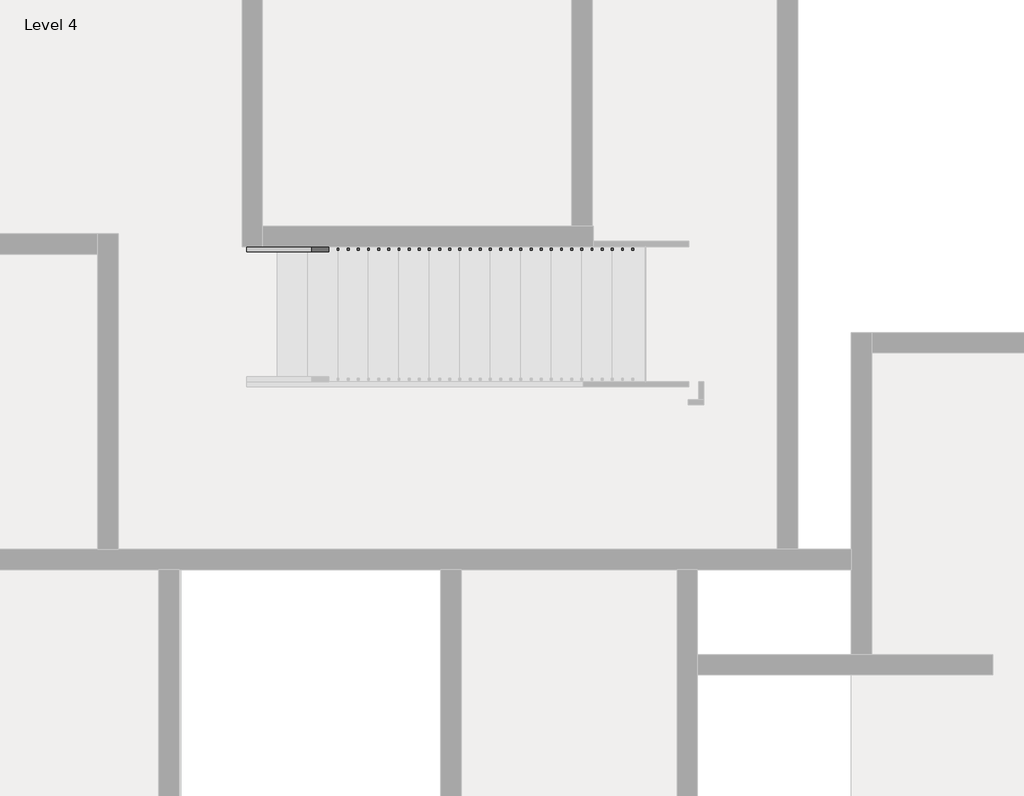
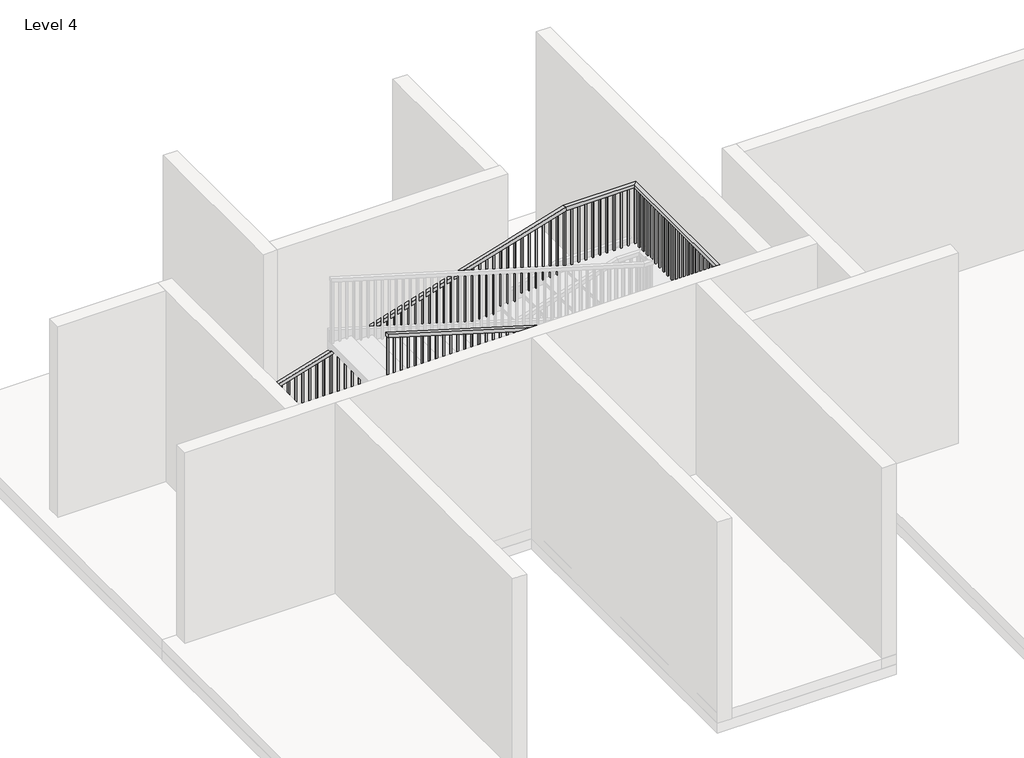
# One storey, part 10 of 14: 1 railing.
"""IFC4 building model written with IfcOpenShell, lengths in millimetres."""

from ifc_helpers import new_model, si_unit, frame, origin, place, context, project, spatial, polyline, outline, extrude, faceted_brep, element, save

model = new_model("IFC4")

# Units and contexts
model_context = context("Model", 3, world=origin())
ifc_project = project(units=[si_unit("LENGTHUNIT", "METRE", prefix="MILLI")], contexts=[model_context])

# Site, building, storey
site = spatial("IfcSite", under=ifc_project)
building = spatial("IfcBuilding", under=site)
storey = spatial("IfcBuildingStorey", under=building, Name="Level 4", Elevation=9144.0)

# Railing
placement = place(None, origin())
element("IfcRailing", 1, ObjectType="Handrail - Rectangular", at=placement, inside=storey, context=model_context, shape_type="SolidModel", body=[
    faceted_brep([(-5254.0891351, 12506.0715905, 10149.84), (-5254.0891351, 12506.0715905, 10096.8032429), (-5254.0891351, 12455.2715905, 10096.8032429), (-5254.0891351, 12455.2715905, 10149.84), (-986.8891351, 12506.0715905, 11430.0), (-979.4332782, 12506.0715905, 11379.2), (-979.4332782, 12455.2715905, 11379.2), (-986.8891351, 12455.2715905, 11430.0), (54.5108649, 12506.0715905, 11430.0), (54.5108649, 12506.0715905, 11379.2), (3.7108649, 12455.2715905, 11379.2), (3.7108649, 12455.2715905, 11430.0), (54.5108649, 9478.4949943, 11430.0), (54.5108649, 9478.4949943, 11379.2), (3.7108649, 9529.2949943, 11379.2), (3.7108649, 9529.2949943, 11430.0), (-682.0891351, 9478.4949943, 11430.0), (-689.544992, 9478.4949943, 11379.2), (-689.544992, 9529.2949943, 11379.2), (-682.0891351, 9529.2949943, 11430.0), (-5254.0891351, 9478.4949943, 12801.6), (-5254.0891351, 9529.2949943, 12801.6), (-5254.0891351, 9529.2949943, 12748.5632429), (-5254.0891351, 9478.4949943, 12748.5632429)], [[[0, 1, 2, 3]], [[1, 0, 4, 5]], [[2, 1, 5, 6]], [[3, 2, 6, 7]], [[0, 3, 7, 4]], [[5, 4, 8, 9]], [[6, 5, 9, 10]], [[7, 6, 10, 11]], [[4, 7, 11, 8]], [[9, 8, 12, 13]], [[10, 9, 13, 14]], [[11, 10, 14, 15]], [[8, 11, 15, 12]], [[13, 12, 16, 17]], [[14, 13, 17, 18]], [[15, 14, 18, 19]], [[12, 15, 19, 16]], [[20, 21, 22, 23]], [[17, 16, 20, 23]], [[18, 17, 23, 22]], [[19, 18, 22, 21]], [[16, 19, 21, 20]]]),
    extrude(outline(polyline([(12720.9407429, -5162.0141351), (11795.76, -5162.0141351), (11795.76, -5142.9641351), (12715.2257429, -5142.9641351), (12720.9407429, -5162.0141351)])), frame((0.0, 9494.3699943, 0.0), z_axis=(0.0, 1.0, 0.0), x_axis=(0.0, 0.0, 1.0)), (0.0, 0.0, 1.0), 19.05),
    extrude(outline(polyline([(12690.4607429, -5060.4141351), (11795.76, -5060.4141351), (11795.76, -5041.3641351), (12684.7457429, -5041.3641351), (12690.4607429, -5060.4141351)])), frame((0.0, 9494.3699943, 0.0), z_axis=(0.0, 1.0, 0.0), x_axis=(0.0, 0.0, 1.0)), (0.0, 0.0, 1.0), 19.05),
    extrude(outline(polyline([(12659.9807429, -4958.8141351), (11795.76, -4958.8141351), (11795.76, -4939.7641351), (12654.2657429, -4939.7641351), (12659.9807429, -4958.8141351)])), frame((0.0, 9494.3699943, 0.0), z_axis=(0.0, 1.0, 0.0), x_axis=(0.0, 0.0, 1.0)), (0.0, 0.0, 1.0), 19.05),
    extrude(outline(polyline([(12629.5007429, -4857.2141351), (11704.32, -4857.2141351), (11704.32, -4838.1641351), (12623.7857429, -4838.1641351), (12629.5007429, -4857.2141351)])), frame((0.0, 9494.3699943, 0.0), z_axis=(0.0, 1.0, 0.0), x_axis=(0.0, 0.0, 1.0)), (0.0, 0.0, 1.0), 19.05),
    extrude(outline(polyline([(12599.0207429, -4755.6141351), (11704.32, -4755.6141351), (11704.32, -4736.5641351), (12593.3057429, -4736.5641351), (12599.0207429, -4755.6141351)])), frame((0.0, 9494.3699943, 0.0), z_axis=(0.0, 1.0, 0.0), x_axis=(0.0, 0.0, 1.0)), (0.0, 0.0, 1.0), 19.05),
    extrude(outline(polyline([(12568.5407429, -4654.0141351), (11704.32, -4654.0141351), (11704.32, -4634.9641351), (12562.8257429, -4634.9641351), (12568.5407429, -4654.0141351)])), frame((0.0, 9494.3699943, 0.0), z_axis=(0.0, 1.0, 0.0), x_axis=(0.0, 0.0, 1.0)), (0.0, 0.0, 1.0), 19.05),
    extrude(outline(polyline([(12538.0607429, -4552.4141351), (11612.88, -4552.4141351), (11612.88, -4533.3641351), (12532.3457429, -4533.3641351), (12538.0607429, -4552.4141351)])), frame((0.0, 9494.3699943, 0.0), z_axis=(0.0, 1.0, 0.0), x_axis=(0.0, 0.0, 1.0)), (0.0, 0.0, 1.0), 19.05),
    extrude(outline(polyline([(12507.5807429, -4450.8141351), (11612.88, -4450.8141351), (11612.88, -4431.7641351), (12501.8657429, -4431.7641351), (12507.5807429, -4450.8141351)])), frame((0.0, 9494.3699943, 0.0), z_axis=(0.0, 1.0, 0.0), x_axis=(0.0, 0.0, 1.0)), (0.0, 0.0, 1.0), 19.05),
    extrude(outline(polyline([(12477.1007429, -4349.2141351), (11612.88, -4349.2141351), (11612.88, -4330.1641351), (12471.3857429, -4330.1641351), (12477.1007429, -4349.2141351)])), frame((0.0, 9494.3699943, 0.0), z_axis=(0.0, 1.0, 0.0), x_axis=(0.0, 0.0, 1.0)), (0.0, 0.0, 1.0), 19.05),
    extrude(outline(polyline([(12446.6207429, -4247.6141351), (11521.44, -4247.6141351), (11521.44, -4228.5641351), (12440.9057429, -4228.5641351), (12446.6207429, -4247.6141351)])), frame((0.0, 9494.3699943, 0.0), z_axis=(0.0, 1.0, 0.0), x_axis=(0.0, 0.0, 1.0)), (0.0, 0.0, 1.0), 19.05),
    extrude(outline(polyline([(12416.1407429, -4146.0141351), (11521.44, -4146.0141351), (11521.44, -4126.9641351), (12410.4257429, -4126.9641351), (12416.1407429, -4146.0141351)])), frame((0.0, 9494.3699943, 0.0), z_axis=(0.0, 1.0, 0.0), x_axis=(0.0, 0.0, 1.0)), (0.0, 0.0, 1.0), 19.05),
    extrude(outline(polyline([(12385.6607429, -4044.4141351), (11521.44, -4044.4141351), (11521.44, -4025.3641351), (12379.9457429, -4025.3641351), (12385.6607429, -4044.4141351)])), frame((0.0, 9494.3699943, 0.0), z_axis=(0.0, 1.0, 0.0), x_axis=(0.0, 0.0, 1.0)), (0.0, 0.0, 1.0), 19.05),
    extrude(outline(polyline([(12355.1807429, -3942.8141351), (11430.0, -3942.8141351), (11430.0, -3923.7641351), (12349.4657429, -3923.7641351), (12355.1807429, -3942.8141351)])), frame((0.0, 9494.3699943, 0.0), z_axis=(0.0, 1.0, 0.0), x_axis=(0.0, 0.0, 1.0)), (0.0, 0.0, 1.0), 19.05),
    extrude(outline(polyline([(12324.7007429, -3841.2141351), (11430.0, -3841.2141351), (11430.0, -3822.1641351), (12318.9857429, -3822.1641351), (12324.7007429, -3841.2141351)])), frame((0.0, 9494.3699943, 0.0), z_axis=(0.0, 1.0, 0.0), x_axis=(0.0, 0.0, 1.0)), (0.0, 0.0, 1.0), 19.05),
    extrude(outline(polyline([(12294.2207429, -3739.6141351), (11430.0, -3739.6141351), (11430.0, -3720.5641351), (12288.5057429, -3720.5641351), (12294.2207429, -3739.6141351)])), frame((0.0, 9494.3699943, 0.0), z_axis=(0.0, 1.0, 0.0), x_axis=(0.0, 0.0, 1.0)), (0.0, 0.0, 1.0), 19.05),
    extrude(outline(polyline([(12263.7407429, -3638.0141351), (11338.56, -3638.0141351), (11338.56, -3618.9641351), (12258.0257429, -3618.9641351), (12263.7407429, -3638.0141351)])), frame((0.0, 9494.3699943, 0.0), z_axis=(0.0, 1.0, 0.0), x_axis=(0.0, 0.0, 1.0)), (0.0, 0.0, 1.0), 19.05),
    extrude(outline(polyline([(12233.2607429, -3536.4141351), (11338.56, -3536.4141351), (11338.56, -3517.3641351), (12227.5457429, -3517.3641351), (12233.2607429, -3536.4141351)])), frame((0.0, 9494.3699943, 0.0), z_axis=(0.0, 1.0, 0.0), x_axis=(0.0, 0.0, 1.0)), (0.0, 0.0, 1.0), 19.05),
    extrude(outline(polyline([(12202.7807429, -3434.8141351), (11338.56, -3434.8141351), (11338.56, -3415.7641351), (12197.0657429, -3415.7641351), (12202.7807429, -3434.8141351)])), frame((0.0, 9494.3699943, 0.0), z_axis=(0.0, 1.0, 0.0), x_axis=(0.0, 0.0, 1.0)), (0.0, 0.0, 1.0), 19.05),
    extrude(outline(polyline([(12172.3007429, -3333.2141351), (11247.12, -3333.2141351), (11247.12, -3314.1641351), (12166.5857429, -3314.1641351), (12172.3007429, -3333.2141351)])), frame((0.0, 9494.3699943, 0.0), z_axis=(0.0, 1.0, 0.0), x_axis=(0.0, 0.0, 1.0)), (0.0, 0.0, 1.0), 19.05),
    extrude(outline(polyline([(12141.8207429, -3231.6141351), (11247.12, -3231.6141351), (11247.12, -3212.5641351), (12136.1057429, -3212.5641351), (12141.8207429, -3231.6141351)])), frame((0.0, 9494.3699943, 0.0), z_axis=(0.0, 1.0, 0.0), x_axis=(0.0, 0.0, 1.0)), (0.0, 0.0, 1.0), 19.05),
    extrude(outline(polyline([(12111.3407429, -3130.0141351), (11247.12, -3130.0141351), (11247.12, -3110.9641351), (12105.6257429, -3110.9641351), (12111.3407429, -3130.0141351)])), frame((0.0, 9494.3699943, 0.0), z_axis=(0.0, 1.0, 0.0), x_axis=(0.0, 0.0, 1.0)), (0.0, 0.0, 1.0), 19.05),
    extrude(outline(polyline([(12080.8607429, -3028.4141351), (11155.68, -3028.4141351), (11155.68, -3009.3641351), (12075.1457429, -3009.3641351), (12080.8607429, -3028.4141351)])), frame((0.0, 9494.3699943, 0.0), z_axis=(0.0, 1.0, 0.0), x_axis=(0.0, 0.0, 1.0)), (0.0, 0.0, 1.0), 19.05),
    extrude(outline(polyline([(12050.3807429, -2926.8141351), (11155.68, -2926.8141351), (11155.68, -2907.7641351), (12044.6657429, -2907.7641351), (12050.3807429, -2926.8141351)])), frame((0.0, 9494.3699943, 0.0), z_axis=(0.0, 1.0, 0.0), x_axis=(0.0, 0.0, 1.0)), (0.0, 0.0, 1.0), 19.05),
    extrude(outline(polyline([(12019.9007429, -2825.2141351), (11155.68, -2825.2141351), (11155.68, -2806.1641351), (12014.1857429, -2806.1641351), (12019.9007429, -2825.2141351)])), frame((0.0, 9494.3699943, 0.0), z_axis=(0.0, 1.0, 0.0), x_axis=(0.0, 0.0, 1.0)), (0.0, 0.0, 1.0), 19.05),
    extrude(outline(polyline([(11989.4207429, -2723.6141351), (11064.24, -2723.6141351), (11064.24, -2704.5641351), (11983.7057429, -2704.5641351), (11989.4207429, -2723.6141351)])), frame((0.0, 9494.3699943, 0.0), z_axis=(0.0, 1.0, 0.0), x_axis=(0.0, 0.0, 1.0)), (0.0, 0.0, 1.0), 19.05),
    extrude(outline(polyline([(11958.9407429, -2622.0141351), (11064.24, -2622.0141351), (11064.24, -2602.9641351), (11953.2257429, -2602.9641351), (11958.9407429, -2622.0141351)])), frame((0.0, 9494.3699943, 0.0), z_axis=(0.0, 1.0, 0.0), x_axis=(0.0, 0.0, 1.0)), (0.0, 0.0, 1.0), 19.05),
    extrude(outline(polyline([(11928.4607429, -2520.4141351), (11064.24, -2520.4141351), (11064.24, -2501.3641351), (11922.7457429, -2501.3641351), (11928.4607429, -2520.4141351)])), frame((0.0, 9494.3699943, 0.0), z_axis=(0.0, 1.0, 0.0), x_axis=(0.0, 0.0, 1.0)), (0.0, 0.0, 1.0), 19.05),
    extrude(outline(polyline([(11897.9807429, -2418.8141351), (10972.8, -2418.8141351), (10972.8, -2399.7641351), (11892.2657429, -2399.7641351), (11897.9807429, -2418.8141351)])), frame((0.0, 9494.3699943, 0.0), z_axis=(0.0, 1.0, 0.0), x_axis=(0.0, 0.0, 1.0)), (0.0, 0.0, 1.0), 19.05),
    extrude(outline(polyline([(11867.5007429, -2317.2141351), (10972.8, -2317.2141351), (10972.8, -2298.1641351), (11861.7857429, -2298.1641351), (11867.5007429, -2317.2141351)])), frame((0.0, 9494.3699943, 0.0), z_axis=(0.0, 1.0, 0.0), x_axis=(0.0, 0.0, 1.0)), (0.0, 0.0, 1.0), 19.05),
    extrude(outline(polyline([(11837.0207429, -2215.6141351), (10972.8, -2215.6141351), (10972.8, -2196.5641351), (11831.3057429, -2196.5641351), (11837.0207429, -2215.6141351)])), frame((0.0, 9494.3699943, 0.0), z_axis=(0.0, 1.0, 0.0), x_axis=(0.0, 0.0, 1.0)), (0.0, 0.0, 1.0), 19.05),
    extrude(outline(polyline([(11806.5407429, -2114.0141351), (10881.36, -2114.0141351), (10881.36, -2094.9641351), (11800.8257429, -2094.9641351), (11806.5407429, -2114.0141351)])), frame((0.0, 9494.3699943, 0.0), z_axis=(0.0, 1.0, 0.0), x_axis=(0.0, 0.0, 1.0)), (0.0, 0.0, 1.0), 19.05),
    extrude(outline(polyline([(11776.0607429, -2012.4141351), (10881.36, -2012.4141351), (10881.36, -1993.3641351), (11770.3457429, -1993.3641351), (11776.0607429, -2012.4141351)])), frame((0.0, 9494.3699943, 0.0), z_axis=(0.0, 1.0, 0.0), x_axis=(0.0, 0.0, 1.0)), (0.0, 0.0, 1.0), 19.05),
    extrude(outline(polyline([(11745.5807429, -1910.8141351), (10881.36, -1910.8141351), (10881.36, -1891.7641351), (11739.8657429, -1891.7641351), (11745.5807429, -1910.8141351)])), frame((0.0, 9494.3699943, 0.0), z_axis=(0.0, 1.0, 0.0), x_axis=(0.0, 0.0, 1.0)), (0.0, 0.0, 1.0), 19.05),
    extrude(outline(polyline([(11715.1007429, -1809.2141351), (10789.92, -1809.2141351), (10789.92, -1790.1641351), (11709.3857429, -1790.1641351), (11715.1007429, -1809.2141351)])), frame((0.0, 9494.3699943, 0.0), z_axis=(0.0, 1.0, 0.0), x_axis=(0.0, 0.0, 1.0)), (0.0, 0.0, 1.0), 19.05),
    extrude(outline(polyline([(11684.6207429, -1707.6141351), (10789.92, -1707.6141351), (10789.92, -1688.5641351), (11678.9057429, -1688.5641351), (11684.6207429, -1707.6141351)])), frame((0.0, 9494.3699943, 0.0), z_axis=(0.0, 1.0, 0.0), x_axis=(0.0, 0.0, 1.0)), (0.0, 0.0, 1.0), 19.05),
    extrude(outline(polyline([(11654.1407429, -1606.0141351), (10789.92, -1606.0141351), (10789.92, -1586.9641351), (11648.4257429, -1586.9641351), (11654.1407429, -1606.0141351)])), frame((0.0, 9494.3699943, 0.0), z_axis=(0.0, 1.0, 0.0), x_axis=(0.0, 0.0, 1.0)), (0.0, 0.0, 1.0), 19.05),
    extrude(outline(polyline([(11623.6607429, -1504.4141351), (10698.48, -1504.4141351), (10698.48, -1485.3641351), (11617.9457429, -1485.3641351), (11623.6607429, -1504.4141351)])), frame((0.0, 9494.3699943, 0.0), z_axis=(0.0, 1.0, 0.0), x_axis=(0.0, 0.0, 1.0)), (0.0, 0.0, 1.0), 19.05),
    extrude(outline(polyline([(11593.1807429, -1402.8141351), (10698.48, -1402.8141351), (10698.48, -1383.7641351), (11587.4657429, -1383.7641351), (11593.1807429, -1402.8141351)])), frame((0.0, 9494.3699943, 0.0), z_axis=(0.0, 1.0, 0.0), x_axis=(0.0, 0.0, 1.0)), (0.0, 0.0, 1.0), 19.05),
    extrude(outline(polyline([(11562.7007429, -1301.2141351), (10698.48, -1301.2141351), (10698.48, -1282.1641351), (11556.9857429, -1282.1641351), (11562.7007429, -1301.2141351)])), frame((0.0, 9494.3699943, 0.0), z_axis=(0.0, 1.0, 0.0), x_axis=(0.0, 0.0, 1.0)), (0.0, 0.0, 1.0), 19.05),
    extrude(outline(polyline([(11532.2207429, -1199.6141351), (10607.04, -1199.6141351), (10607.04, -1180.5641351), (11526.5057429, -1180.5641351), (11532.2207429, -1199.6141351)])), frame((0.0, 9494.3699943, 0.0), z_axis=(0.0, 1.0, 0.0), x_axis=(0.0, 0.0, 1.0)), (0.0, 0.0, 1.0), 19.05),
    extrude(outline(polyline([(11501.7407429, -1098.0141351), (10607.04, -1098.0141351), (10607.04, -1078.9641351), (11496.0257429, -1078.9641351), (11501.7407429, -1098.0141351)])), frame((0.0, 9494.3699943, 0.0), z_axis=(0.0, 1.0, 0.0), x_axis=(0.0, 0.0, 1.0)), (0.0, 0.0, 1.0), 19.05),
    extrude(outline(polyline([(11471.2607429, -996.4141351), (10607.04, -996.4141351), (10607.04, -977.3641351), (11465.5457429, -977.3641351), (11471.2607429, -996.4141351)])), frame((0.0, 9494.3699943, 0.0), z_axis=(0.0, 1.0, 0.0), x_axis=(0.0, 0.0, 1.0)), (0.0, 0.0, 1.0), 19.05),
    extrude(outline(polyline([(11440.7807429, -894.8141351), (10515.6, -894.8141351), (10515.6, -875.7641351), (11435.0657429, -875.7641351), (11440.7807429, -894.8141351)])), frame((0.0, 9494.3699943, 0.0), z_axis=(0.0, 1.0, 0.0), x_axis=(0.0, 0.0, 1.0)), (0.0, 0.0, 1.0), 19.05),
    extrude(outline(polyline([(11410.3007429, -793.2141351), (10515.6, -793.2141351), (10515.6, -774.1641351), (11404.5857429, -774.1641351), (11410.3007429, -793.2141351)])), frame((0.0, 9494.3699943, 0.0), z_axis=(0.0, 1.0, 0.0), x_axis=(0.0, 0.0, 1.0)), (0.0, 0.0, 1.0), 19.05),
    extrude(outline(polyline([(-672.5641351, 9494.3699943), (-691.6141351, 9494.3699943), (-691.6141351, 9513.4199943), (-672.5641351, 9513.4199943), (-672.5641351, 9494.3699943)])), frame((0.0, 0.0, 10515.6), z_axis=(0.0, 0.0, 1.0), x_axis=(1.0, 0.0, 0.0)), (0.0, 0.0, 1.0), 863.6),
    extrude(outline(polyline([(-570.9641351, 9494.3699943), (-590.0141351, 9494.3699943), (-590.0141351, 9513.4199943), (-570.9641351, 9513.4199943), (-570.9641351, 9494.3699943)])), frame((0.0, 0.0, 10515.6), z_axis=(0.0, 0.0, 1.0), x_axis=(1.0, 0.0, 0.0)), (0.0, 0.0, 1.0), 863.6),
    extrude(outline(polyline([(-469.3641351, 9494.3699943), (-488.4141351, 9494.3699943), (-488.4141351, 9513.4199943), (-469.3641351, 9513.4199943), (-469.3641351, 9494.3699943)])), frame((0.0, 0.0, 10515.6), z_axis=(0.0, 0.0, 1.0), x_axis=(1.0, 0.0, 0.0)), (0.0, 0.0, 1.0), 863.6),
    extrude(outline(polyline([(-367.7641351, 9494.3699943), (-386.8141351, 9494.3699943), (-386.8141351, 9513.4199943), (-367.7641351, 9513.4199943), (-367.7641351, 9494.3699943)])), frame((0.0, 0.0, 10515.6), z_axis=(0.0, 0.0, 1.0), x_axis=(1.0, 0.0, 0.0)), (0.0, 0.0, 1.0), 863.6),
    extrude(outline(polyline([(-266.1641351, 9494.3699943), (-285.2141351, 9494.3699943), (-285.2141351, 9513.4199943), (-266.1641351, 9513.4199943), (-266.1641351, 9494.3699943)])), frame((0.0, 0.0, 10515.6), z_axis=(0.0, 0.0, 1.0), x_axis=(1.0, 0.0, 0.0)), (0.0, 0.0, 1.0), 863.6),
    extrude(outline(polyline([(-164.5641351, 9494.3699943), (-183.6141351, 9494.3699943), (-183.6141351, 9513.4199943), (-164.5641351, 9513.4199943), (-164.5641351, 9494.3699943)])), frame((0.0, 0.0, 10515.6), z_axis=(0.0, 0.0, 1.0), x_axis=(1.0, 0.0, 0.0)), (0.0, 0.0, 1.0), 863.6),
    extrude(outline(polyline([(-62.9641351, 9494.3699943), (-82.0141351, 9494.3699943), (-82.0141351, 9513.4199943), (-62.9641351, 9513.4199943), (-62.9641351, 9494.3699943)])), frame((0.0, 0.0, 10515.6), z_axis=(0.0, 0.0, 1.0), x_axis=(1.0, 0.0, 0.0)), (0.0, 0.0, 1.0), 863.6),
    extrude(outline(polyline([(38.6358649, 9543.7965905), (38.6358649, 9524.7465905), (19.5858649, 9524.7465905), (19.5858649, 9543.7965905), (38.6358649, 9543.7965905)])), frame((0.0, 0.0, 10515.6), z_axis=(0.0, 0.0, 1.0), x_axis=(1.0, 0.0, 0.0)), (0.0, 0.0, 1.0), 863.6),
    extrude(outline(polyline([(38.6358649, 9645.3965905), (38.6358649, 9626.3465905), (19.5858649, 9626.3465905), (19.5858649, 9645.3965905), (38.6358649, 9645.3965905)])), frame((0.0, 0.0, 10515.6), z_axis=(0.0, 0.0, 1.0), x_axis=(1.0, 0.0, 0.0)), (0.0, 0.0, 1.0), 863.6),
    extrude(outline(polyline([(38.6358649, 9746.9965905), (38.6358649, 9727.9465905), (19.5858649, 9727.9465905), (19.5858649, 9746.9965905), (38.6358649, 9746.9965905)])), frame((0.0, 0.0, 10515.6), z_axis=(0.0, 0.0, 1.0), x_axis=(1.0, 0.0, 0.0)), (0.0, 0.0, 1.0), 863.6),
    extrude(outline(polyline([(38.6358649, 9848.5965905), (38.6358649, 9829.5465905), (19.5858649, 9829.5465905), (19.5858649, 9848.5965905), (38.6358649, 9848.5965905)])), frame((0.0, 0.0, 10515.6), z_axis=(0.0, 0.0, 1.0), x_axis=(1.0, 0.0, 0.0)), (0.0, 0.0, 1.0), 863.6),
    extrude(outline(polyline([(38.6358649, 9950.1965905), (38.6358649, 9931.1465905), (19.5858649, 9931.1465905), (19.5858649, 9950.1965905), (38.6358649, 9950.1965905)])), frame((0.0, 0.0, 10515.6), z_axis=(0.0, 0.0, 1.0), x_axis=(1.0, 0.0, 0.0)), (0.0, 0.0, 1.0), 863.6),
    extrude(outline(polyline([(38.6358649, 10051.7965905), (38.6358649, 10032.7465905), (19.5858649, 10032.7465905), (19.5858649, 10051.7965905), (38.6358649, 10051.7965905)])), frame((0.0, 0.0, 10515.6), z_axis=(0.0, 0.0, 1.0), x_axis=(1.0, 0.0, 0.0)), (0.0, 0.0, 1.0), 863.6),
    extrude(outline(polyline([(38.6358649, 10153.3965905), (38.6358649, 10134.3465905), (19.5858649, 10134.3465905), (19.5858649, 10153.3965905), (38.6358649, 10153.3965905)])), frame((0.0, 0.0, 10515.6), z_axis=(0.0, 0.0, 1.0), x_axis=(1.0, 0.0, 0.0)), (0.0, 0.0, 1.0), 863.6),
    extrude(outline(polyline([(38.6358649, 10254.9965905), (38.6358649, 10235.9465905), (19.5858649, 10235.9465905), (19.5858649, 10254.9965905), (38.6358649, 10254.9965905)])), frame((0.0, 0.0, 10515.6), z_axis=(0.0, 0.0, 1.0), x_axis=(1.0, 0.0, 0.0)), (0.0, 0.0, 1.0), 863.6),
    extrude(outline(polyline([(38.6358649, 10356.5965905), (38.6358649, 10337.5465905), (19.5858649, 10337.5465905), (19.5858649, 10356.5965905), (38.6358649, 10356.5965905)])), frame((0.0, 0.0, 10515.6), z_axis=(0.0, 0.0, 1.0), x_axis=(1.0, 0.0, 0.0)), (0.0, 0.0, 1.0), 863.6),
    extrude(outline(polyline([(38.6358649, 10458.1965905), (38.6358649, 10439.1465905), (19.5858649, 10439.1465905), (19.5858649, 10458.1965905), (38.6358649, 10458.1965905)])), frame((0.0, 0.0, 10515.6), z_axis=(0.0, 0.0, 1.0), x_axis=(1.0, 0.0, 0.0)), (0.0, 0.0, 1.0), 863.6),
    extrude(outline(polyline([(38.6358649, 10559.7965905), (38.6358649, 10540.7465905), (19.5858649, 10540.7465905), (19.5858649, 10559.7965905), (38.6358649, 10559.7965905)])), frame((0.0, 0.0, 10515.6), z_axis=(0.0, 0.0, 1.0), x_axis=(1.0, 0.0, 0.0)), (0.0, 0.0, 1.0), 863.6),
    extrude(outline(polyline([(38.6358649, 10661.3965905), (38.6358649, 10642.3465905), (19.5858649, 10642.3465905), (19.5858649, 10661.3965905), (38.6358649, 10661.3965905)])), frame((0.0, 0.0, 10515.6), z_axis=(0.0, 0.0, 1.0), x_axis=(1.0, 0.0, 0.0)), (0.0, 0.0, 1.0), 863.6),
    extrude(outline(polyline([(38.6358649, 10762.9965905), (38.6358649, 10743.9465905), (19.5858649, 10743.9465905), (19.5858649, 10762.9965905), (38.6358649, 10762.9965905)])), frame((0.0, 0.0, 10515.6), z_axis=(0.0, 0.0, 1.0), x_axis=(1.0, 0.0, 0.0)), (0.0, 0.0, 1.0), 863.6),
    extrude(outline(polyline([(38.6358649, 10864.5965905), (38.6358649, 10845.5465905), (19.5858649, 10845.5465905), (19.5858649, 10864.5965905), (38.6358649, 10864.5965905)])), frame((0.0, 0.0, 10515.6), z_axis=(0.0, 0.0, 1.0), x_axis=(1.0, 0.0, 0.0)), (0.0, 0.0, 1.0), 863.6),
    extrude(outline(polyline([(38.6358649, 10966.1965905), (38.6358649, 10947.1465905), (19.5858649, 10947.1465905), (19.5858649, 10966.1965905), (38.6358649, 10966.1965905)])), frame((0.0, 0.0, 10515.6), z_axis=(0.0, 0.0, 1.0), x_axis=(1.0, 0.0, 0.0)), (0.0, 0.0, 1.0), 863.6),
    extrude(outline(polyline([(38.6358649, 11067.7965905), (38.6358649, 11048.7465905), (19.5858649, 11048.7465905), (19.5858649, 11067.7965905), (38.6358649, 11067.7965905)])), frame((0.0, 0.0, 10515.6), z_axis=(0.0, 0.0, 1.0), x_axis=(1.0, 0.0, 0.0)), (0.0, 0.0, 1.0), 863.6),
    extrude(outline(polyline([(38.6358649, 11169.3965905), (38.6358649, 11150.3465905), (19.5858649, 11150.3465905), (19.5858649, 11169.3965905), (38.6358649, 11169.3965905)])), frame((0.0, 0.0, 10515.6), z_axis=(0.0, 0.0, 1.0), x_axis=(1.0, 0.0, 0.0)), (0.0, 0.0, 1.0), 863.6),
    extrude(outline(polyline([(38.6358649, 11270.9965905), (38.6358649, 11251.9465905), (19.5858649, 11251.9465905), (19.5858649, 11270.9965905), (38.6358649, 11270.9965905)])), frame((0.0, 0.0, 10515.6), z_axis=(0.0, 0.0, 1.0), x_axis=(1.0, 0.0, 0.0)), (0.0, 0.0, 1.0), 863.6),
    extrude(outline(polyline([(38.6358649, 11372.5965905), (38.6358649, 11353.5465905), (19.5858649, 11353.5465905), (19.5858649, 11372.5965905), (38.6358649, 11372.5965905)])), frame((0.0, 0.0, 10515.6), z_axis=(0.0, 0.0, 1.0), x_axis=(1.0, 0.0, 0.0)), (0.0, 0.0, 1.0), 863.6),
    extrude(outline(polyline([(38.6358649, 11474.1965905), (38.6358649, 11455.1465905), (19.5858649, 11455.1465905), (19.5858649, 11474.1965905), (38.6358649, 11474.1965905)])), frame((0.0, 0.0, 10515.6), z_axis=(0.0, 0.0, 1.0), x_axis=(1.0, 0.0, 0.0)), (0.0, 0.0, 1.0), 863.6),
    extrude(outline(polyline([(38.6358649, 11575.7965905), (38.6358649, 11556.7465905), (19.5858649, 11556.7465905), (19.5858649, 11575.7965905), (38.6358649, 11575.7965905)])), frame((0.0, 0.0, 10515.6), z_axis=(0.0, 0.0, 1.0), x_axis=(1.0, 0.0, 0.0)), (0.0, 0.0, 1.0), 863.6),
    extrude(outline(polyline([(38.6358649, 11677.3965905), (38.6358649, 11658.3465905), (19.5858649, 11658.3465905), (19.5858649, 11677.3965905), (38.6358649, 11677.3965905)])), frame((0.0, 0.0, 10515.6), z_axis=(0.0, 0.0, 1.0), x_axis=(1.0, 0.0, 0.0)), (0.0, 0.0, 1.0), 863.6),
    extrude(outline(polyline([(38.6358649, 11778.9965905), (38.6358649, 11759.9465905), (19.5858649, 11759.9465905), (19.5858649, 11778.9965905), (38.6358649, 11778.9965905)])), frame((0.0, 0.0, 10515.6), z_axis=(0.0, 0.0, 1.0), x_axis=(1.0, 0.0, 0.0)), (0.0, 0.0, 1.0), 863.6),
    extrude(outline(polyline([(38.6358649, 11880.5965905), (38.6358649, 11861.5465905), (19.5858649, 11861.5465905), (19.5858649, 11880.5965905), (38.6358649, 11880.5965905)])), frame((0.0, 0.0, 10515.6), z_axis=(0.0, 0.0, 1.0), x_axis=(1.0, 0.0, 0.0)), (0.0, 0.0, 1.0), 863.6),
    extrude(outline(polyline([(38.6358649, 11982.1965905), (38.6358649, 11963.1465905), (19.5858649, 11963.1465905), (19.5858649, 11982.1965905), (38.6358649, 11982.1965905)])), frame((0.0, 0.0, 10515.6), z_axis=(0.0, 0.0, 1.0), x_axis=(1.0, 0.0, 0.0)), (0.0, 0.0, 1.0), 863.6),
    extrude(outline(polyline([(38.6358649, 12083.7965905), (38.6358649, 12064.7465905), (19.5858649, 12064.7465905), (19.5858649, 12083.7965905), (38.6358649, 12083.7965905)])), frame((0.0, 0.0, 10515.6), z_axis=(0.0, 0.0, 1.0), x_axis=(1.0, 0.0, 0.0)), (0.0, 0.0, 1.0), 863.6),
    extrude(outline(polyline([(38.6358649, 12185.3965905), (38.6358649, 12166.3465905), (19.5858649, 12166.3465905), (19.5858649, 12185.3965905), (38.6358649, 12185.3965905)])), frame((0.0, 0.0, 10515.6), z_axis=(0.0, 0.0, 1.0), x_axis=(1.0, 0.0, 0.0)), (0.0, 0.0, 1.0), 863.6),
    extrude(outline(polyline([(38.6358649, 12286.9965905), (38.6358649, 12267.9465905), (19.5858649, 12267.9465905), (19.5858649, 12286.9965905), (38.6358649, 12286.9965905)])), frame((0.0, 0.0, 10515.6), z_axis=(0.0, 0.0, 1.0), x_axis=(1.0, 0.0, 0.0)), (0.0, 0.0, 1.0), 863.6),
    extrude(outline(polyline([(38.6358649, 12388.5965905), (38.6358649, 12369.5465905), (19.5858649, 12369.5465905), (19.5858649, 12388.5965905), (38.6358649, 12388.5965905)])), frame((0.0, 0.0, 10515.6), z_axis=(0.0, 0.0, 1.0), x_axis=(1.0, 0.0, 0.0)), (0.0, 0.0, 1.0), 863.6),
    extrude(outline(polyline([(-82.0141351, 12490.1965905), (-62.9641351, 12490.1965905), (-62.9641351, 12471.1465905), (-82.0141351, 12471.1465905), (-82.0141351, 12490.1965905)])), frame((0.0, 0.0, 10515.6), z_axis=(0.0, 0.0, 1.0), x_axis=(1.0, 0.0, 0.0)), (0.0, 0.0, 1.0), 863.6),
    extrude(outline(polyline([(-183.6141351, 12490.1965905), (-164.5641351, 12490.1965905), (-164.5641351, 12471.1465905), (-183.6141351, 12471.1465905), (-183.6141351, 12490.1965905)])), frame((0.0, 0.0, 10515.6), z_axis=(0.0, 0.0, 1.0), x_axis=(1.0, 0.0, 0.0)), (0.0, 0.0, 1.0), 863.6),
    extrude(outline(polyline([(-285.2141351, 12490.1965905), (-266.1641351, 12490.1965905), (-266.1641351, 12471.1465905), (-285.2141351, 12471.1465905), (-285.2141351, 12490.1965905)])), frame((0.0, 0.0, 10515.6), z_axis=(0.0, 0.0, 1.0), x_axis=(1.0, 0.0, 0.0)), (0.0, 0.0, 1.0), 863.6),
    extrude(outline(polyline([(-386.8141351, 12490.1965905), (-367.7641351, 12490.1965905), (-367.7641351, 12471.1465905), (-386.8141351, 12471.1465905), (-386.8141351, 12490.1965905)])), frame((0.0, 0.0, 10515.6), z_axis=(0.0, 0.0, 1.0), x_axis=(1.0, 0.0, 0.0)), (0.0, 0.0, 1.0), 863.6),
    extrude(outline(polyline([(-488.4141351, 12490.1965905), (-469.3641351, 12490.1965905), (-469.3641351, 12471.1465905), (-488.4141351, 12471.1465905), (-488.4141351, 12490.1965905)])), frame((0.0, 0.0, 10515.6), z_axis=(0.0, 0.0, 1.0), x_axis=(1.0, 0.0, 0.0)), (0.0, 0.0, 1.0), 863.6),
    extrude(outline(polyline([(-590.0141351, 12490.1965905), (-570.9641351, 12490.1965905), (-570.9641351, 12471.1465905), (-590.0141351, 12471.1465905), (-590.0141351, 12490.1965905)])), frame((0.0, 0.0, 10515.6), z_axis=(0.0, 0.0, 1.0), x_axis=(1.0, 0.0, 0.0)), (0.0, 0.0, 1.0), 863.6),
    extrude(outline(polyline([(-691.6141351, 12490.1965905), (-672.5641351, 12490.1965905), (-672.5641351, 12471.1465905), (-691.6141351, 12471.1465905), (-691.6141351, 12490.1965905)])), frame((0.0, 0.0, 10515.6), z_axis=(0.0, 0.0, 1.0), x_axis=(1.0, 0.0, 0.0)), (0.0, 0.0, 1.0), 863.6),
    extrude(outline(polyline([(-793.2141351, 12490.1965905), (-774.1641351, 12490.1965905), (-774.1641351, 12471.1465905), (-793.2141351, 12471.1465905), (-793.2141351, 12490.1965905)])), frame((0.0, 0.0, 10515.6), z_axis=(0.0, 0.0, 1.0), x_axis=(1.0, 0.0, 0.0)), (0.0, 0.0, 1.0), 863.6),
    extrude(outline(polyline([(-894.8141351, 12490.1965905), (-875.7641351, 12490.1965905), (-875.7641351, 12471.1465905), (-894.8141351, 12471.1465905), (-894.8141351, 12490.1965905)])), frame((0.0, 0.0, 10515.6), z_axis=(0.0, 0.0, 1.0), x_axis=(1.0, 0.0, 0.0)), (0.0, 0.0, 1.0), 863.6),
    extrude(outline(polyline([(11374.1057429, -996.4141351), (10515.6, -996.4141351), (10515.6, -977.3641351), (11379.8207429, -977.3641351), (11374.1057429, -996.4141351)])), frame((0.0, 12471.1465905, 0.0), z_axis=(0.0, 1.0, 0.0), x_axis=(0.0, 0.0, 1.0)), (0.0, 0.0, 1.0), 19.05),
    extrude(outline(polyline([(11343.6257429, -1098.0141351), (10424.16, -1098.0141351), (10424.16, -1078.9641351), (11349.3407429, -1078.9641351), (11343.6257429, -1098.0141351)])), frame((0.0, 12471.1465905, 0.0), z_axis=(0.0, 1.0, 0.0), x_axis=(0.0, 0.0, 1.0)), (0.0, 0.0, 1.0), 19.05),
    extrude(outline(polyline([(11313.1457429, -1199.6141351), (10424.16, -1199.6141351), (10424.16, -1180.5641351), (11318.8607429, -1180.5641351), (11313.1457429, -1199.6141351)])), frame((0.0, 12471.1465905, 0.0), z_axis=(0.0, 1.0, 0.0), x_axis=(0.0, 0.0, 1.0)), (0.0, 0.0, 1.0), 19.05),
    extrude(outline(polyline([(11282.6657429, -1301.2141351), (10424.16, -1301.2141351), (10424.16, -1282.1641351), (11288.3807429, -1282.1641351), (11282.6657429, -1301.2141351)])), frame((0.0, 12471.1465905, 0.0), z_axis=(0.0, 1.0, 0.0), x_axis=(0.0, 0.0, 1.0)), (0.0, 0.0, 1.0), 19.05),
    extrude(outline(polyline([(11252.1857429, -1402.8141351), (10332.72, -1402.8141351), (10332.72, -1383.7641351), (11257.9007429, -1383.7641351), (11252.1857429, -1402.8141351)])), frame((0.0, 12471.1465905, 0.0), z_axis=(0.0, 1.0, 0.0), x_axis=(0.0, 0.0, 1.0)), (0.0, 0.0, 1.0), 19.05),
    extrude(outline(polyline([(11221.7057429, -1504.4141351), (10332.72, -1504.4141351), (10332.72, -1485.3641351), (11227.4207429, -1485.3641351), (11221.7057429, -1504.4141351)])), frame((0.0, 12471.1465905, 0.0), z_axis=(0.0, 1.0, 0.0), x_axis=(0.0, 0.0, 1.0)), (0.0, 0.0, 1.0), 19.05),
    extrude(outline(polyline([(11191.2257429, -1606.0141351), (10332.72, -1606.0141351), (10332.72, -1586.9641351), (11196.9407429, -1586.9641351), (11191.2257429, -1606.0141351)])), frame((0.0, 12471.1465905, 0.0), z_axis=(0.0, 1.0, 0.0), x_axis=(0.0, 0.0, 1.0)), (0.0, 0.0, 1.0), 19.05),
    extrude(outline(polyline([(11160.7457429, -1707.6141351), (10241.28, -1707.6141351), (10241.28, -1688.5641351), (11166.4607429, -1688.5641351), (11160.7457429, -1707.6141351)])), frame((0.0, 12471.1465905, 0.0), z_axis=(0.0, 1.0, 0.0), x_axis=(0.0, 0.0, 1.0)), (0.0, 0.0, 1.0), 19.05),
    extrude(outline(polyline([(11130.2657429, -1809.2141351), (10241.28, -1809.2141351), (10241.28, -1790.1641351), (11135.9807429, -1790.1641351), (11130.2657429, -1809.2141351)])), frame((0.0, 12471.1465905, 0.0), z_axis=(0.0, 1.0, 0.0), x_axis=(0.0, 0.0, 1.0)), (0.0, 0.0, 1.0), 19.05),
    extrude(outline(polyline([(11099.7857429, -1910.8141351), (10241.28, -1910.8141351), (10241.28, -1891.7641351), (11105.5007429, -1891.7641351), (11099.7857429, -1910.8141351)])), frame((0.0, 12471.1465905, 0.0), z_axis=(0.0, 1.0, 0.0), x_axis=(0.0, 0.0, 1.0)), (0.0, 0.0, 1.0), 19.05),
    extrude(outline(polyline([(11069.3057429, -2012.4141351), (10149.84, -2012.4141351), (10149.84, -1993.3641351), (11075.0207429, -1993.3641351), (11069.3057429, -2012.4141351)])), frame((0.0, 12471.1465905, 0.0), z_axis=(0.0, 1.0, 0.0), x_axis=(0.0, 0.0, 1.0)), (0.0, 0.0, 1.0), 19.05),
    extrude(outline(polyline([(11038.8257429, -2114.0141351), (10149.84, -2114.0141351), (10149.84, -2094.9641351), (11044.5407429, -2094.9641351), (11038.8257429, -2114.0141351)])), frame((0.0, 12471.1465905, 0.0), z_axis=(0.0, 1.0, 0.0), x_axis=(0.0, 0.0, 1.0)), (0.0, 0.0, 1.0), 19.05),
    extrude(outline(polyline([(11008.3457429, -2215.6141351), (10149.84, -2215.6141351), (10149.84, -2196.5641351), (11014.0607429, -2196.5641351), (11008.3457429, -2215.6141351)])), frame((0.0, 12471.1465905, 0.0), z_axis=(0.0, 1.0, 0.0), x_axis=(0.0, 0.0, 1.0)), (0.0, 0.0, 1.0), 19.05),
    extrude(outline(polyline([(10977.8657429, -2317.2141351), (10058.4, -2317.2141351), (10058.4, -2298.1641351), (10983.5807429, -2298.1641351), (10977.8657429, -2317.2141351)])), frame((0.0, 12471.1465905, 0.0), z_axis=(0.0, 1.0, 0.0), x_axis=(0.0, 0.0, 1.0)), (0.0, 0.0, 1.0), 19.05),
    extrude(outline(polyline([(10947.3857429, -2418.8141351), (10058.4, -2418.8141351), (10058.4, -2399.7641351), (10953.1007429, -2399.7641351), (10947.3857429, -2418.8141351)])), frame((0.0, 12471.1465905, 0.0), z_axis=(0.0, 1.0, 0.0), x_axis=(0.0, 0.0, 1.0)), (0.0, 0.0, 1.0), 19.05),
    extrude(outline(polyline([(10916.9057429, -2520.4141351), (10058.4, -2520.4141351), (10058.4, -2501.3641351), (10922.6207429, -2501.3641351), (10916.9057429, -2520.4141351)])), frame((0.0, 12471.1465905, 0.0), z_axis=(0.0, 1.0, 0.0), x_axis=(0.0, 0.0, 1.0)), (0.0, 0.0, 1.0), 19.05),
    extrude(outline(polyline([(10886.4257429, -2622.0141351), (9966.96, -2622.0141351), (9966.96, -2602.9641351), (10892.1407429, -2602.9641351), (10886.4257429, -2622.0141351)])), frame((0.0, 12471.1465905, 0.0), z_axis=(0.0, 1.0, 0.0), x_axis=(0.0, 0.0, 1.0)), (0.0, 0.0, 1.0), 19.05),
    extrude(outline(polyline([(10855.9457429, -2723.6141351), (9966.96, -2723.6141351), (9966.96, -2704.5641351), (10861.6607429, -2704.5641351), (10855.9457429, -2723.6141351)])), frame((0.0, 12471.1465905, 0.0), z_axis=(0.0, 1.0, 0.0), x_axis=(0.0, 0.0, 1.0)), (0.0, 0.0, 1.0), 19.05),
    extrude(outline(polyline([(10825.4657429, -2825.2141351), (9966.96, -2825.2141351), (9966.96, -2806.1641351), (10831.1807429, -2806.1641351), (10825.4657429, -2825.2141351)])), frame((0.0, 12471.1465905, 0.0), z_axis=(0.0, 1.0, 0.0), x_axis=(0.0, 0.0, 1.0)), (0.0, 0.0, 1.0), 19.05),
    extrude(outline(polyline([(10794.9857429, -2926.8141351), (9875.52, -2926.8141351), (9875.52, -2907.7641351), (10800.7007429, -2907.7641351), (10794.9857429, -2926.8141351)])), frame((0.0, 12471.1465905, 0.0), z_axis=(0.0, 1.0, 0.0), x_axis=(0.0, 0.0, 1.0)), (0.0, 0.0, 1.0), 19.05),
    extrude(outline(polyline([(10764.5057429, -3028.4141351), (9875.52, -3028.4141351), (9875.52, -3009.3641351), (10770.2207429, -3009.3641351), (10764.5057429, -3028.4141351)])), frame((0.0, 12471.1465905, 0.0), z_axis=(0.0, 1.0, 0.0), x_axis=(0.0, 0.0, 1.0)), (0.0, 0.0, 1.0), 19.05),
    extrude(outline(polyline([(10734.0257429, -3130.0141351), (9875.52, -3130.0141351), (9875.52, -3110.9641351), (10739.7407429, -3110.9641351), (10734.0257429, -3130.0141351)])), frame((0.0, 12471.1465905, 0.0), z_axis=(0.0, 1.0, 0.0), x_axis=(0.0, 0.0, 1.0)), (0.0, 0.0, 1.0), 19.05),
    extrude(outline(polyline([(10703.5457429, -3231.6141351), (9784.08, -3231.6141351), (9784.08, -3212.5641351), (10709.2607429, -3212.5641351), (10703.5457429, -3231.6141351)])), frame((0.0, 12471.1465905, 0.0), z_axis=(0.0, 1.0, 0.0), x_axis=(0.0, 0.0, 1.0)), (0.0, 0.0, 1.0), 19.05),
    extrude(outline(polyline([(10673.0657429, -3333.2141351), (9784.08, -3333.2141351), (9784.08, -3314.1641351), (10678.7807429, -3314.1641351), (10673.0657429, -3333.2141351)])), frame((0.0, 12471.1465905, 0.0), z_axis=(0.0, 1.0, 0.0), x_axis=(0.0, 0.0, 1.0)), (0.0, 0.0, 1.0), 19.05),
    extrude(outline(polyline([(10642.5857429, -3434.8141351), (9784.08, -3434.8141351), (9784.08, -3415.7641351), (10648.3007429, -3415.7641351), (10642.5857429, -3434.8141351)])), frame((0.0, 12471.1465905, 0.0), z_axis=(0.0, 1.0, 0.0), x_axis=(0.0, 0.0, 1.0)), (0.0, 0.0, 1.0), 19.05),
    extrude(outline(polyline([(10612.1057429, -3536.4141351), (9692.64, -3536.4141351), (9692.64, -3517.3641351), (10617.8207429, -3517.3641351), (10612.1057429, -3536.4141351)])), frame((0.0, 12471.1465905, 0.0), z_axis=(0.0, 1.0, 0.0), x_axis=(0.0, 0.0, 1.0)), (0.0, 0.0, 1.0), 19.05),
    extrude(outline(polyline([(10581.6257429, -3638.0141351), (9692.64, -3638.0141351), (9692.64, -3618.9641351), (10587.3407429, -3618.9641351), (10581.6257429, -3638.0141351)])), frame((0.0, 12471.1465905, 0.0), z_axis=(0.0, 1.0, 0.0), x_axis=(0.0, 0.0, 1.0)), (0.0, 0.0, 1.0), 19.05),
    extrude(outline(polyline([(10551.1457429, -3739.6141351), (9692.64, -3739.6141351), (9692.64, -3720.5641351), (10556.8607429, -3720.5641351), (10551.1457429, -3739.6141351)])), frame((0.0, 12471.1465905, 0.0), z_axis=(0.0, 1.0, 0.0), x_axis=(0.0, 0.0, 1.0)), (0.0, 0.0, 1.0), 19.05),
    extrude(outline(polyline([(10520.6657429, -3841.2141351), (9601.2, -3841.2141351), (9601.2, -3822.1641351), (10526.3807429, -3822.1641351), (10520.6657429, -3841.2141351)])), frame((0.0, 12471.1465905, 0.0), z_axis=(0.0, 1.0, 0.0), x_axis=(0.0, 0.0, 1.0)), (0.0, 0.0, 1.0), 19.05),
    extrude(outline(polyline([(10490.1857429, -3942.8141351), (9601.2, -3942.8141351), (9601.2, -3923.7641351), (10495.9007429, -3923.7641351), (10490.1857429, -3942.8141351)])), frame((0.0, 12471.1465905, 0.0), z_axis=(0.0, 1.0, 0.0), x_axis=(0.0, 0.0, 1.0)), (0.0, 0.0, 1.0), 19.05),
    extrude(outline(polyline([(10459.7057429, -4044.4141351), (9601.2, -4044.4141351), (9601.2, -4025.3641351), (10465.4207429, -4025.3641351), (10459.7057429, -4044.4141351)])), frame((0.0, 12471.1465905, 0.0), z_axis=(0.0, 1.0, 0.0), x_axis=(0.0, 0.0, 1.0)), (0.0, 0.0, 1.0), 19.05),
    extrude(outline(polyline([(10429.2257429, -4146.0141351), (9509.76, -4146.0141351), (9509.76, -4126.9641351), (10434.9407429, -4126.9641351), (10429.2257429, -4146.0141351)])), frame((0.0, 12471.1465905, 0.0), z_axis=(0.0, 1.0, 0.0), x_axis=(0.0, 0.0, 1.0)), (0.0, 0.0, 1.0), 19.05),
    extrude(outline(polyline([(10398.7457429, -4247.6141351), (9509.76, -4247.6141351), (9509.76, -4228.5641351), (10404.4607429, -4228.5641351), (10398.7457429, -4247.6141351)])), frame((0.0, 12471.1465905, 0.0), z_axis=(0.0, 1.0, 0.0), x_axis=(0.0, 0.0, 1.0)), (0.0, 0.0, 1.0), 19.05),
    extrude(outline(polyline([(10368.2657429, -4349.2141351), (9509.76, -4349.2141351), (9509.76, -4330.1641351), (10373.9807429, -4330.1641351), (10368.2657429, -4349.2141351)])), frame((0.0, 12471.1465905, 0.0), z_axis=(0.0, 1.0, 0.0), x_axis=(0.0, 0.0, 1.0)), (0.0, 0.0, 1.0), 19.05),
    extrude(outline(polyline([(10337.7857429, -4450.8141351), (9418.32, -4450.8141351), (9418.32, -4431.7641351), (10343.5007429, -4431.7641351), (10337.7857429, -4450.8141351)])), frame((0.0, 12471.1465905, 0.0), z_axis=(0.0, 1.0, 0.0), x_axis=(0.0, 0.0, 1.0)), (0.0, 0.0, 1.0), 19.05),
    extrude(outline(polyline([(10307.3057429, -4552.4141351), (9418.32, -4552.4141351), (9418.32, -4533.3641351), (10313.0207429, -4533.3641351), (10307.3057429, -4552.4141351)])), frame((0.0, 12471.1465905, 0.0), z_axis=(0.0, 1.0, 0.0), x_axis=(0.0, 0.0, 1.0)), (0.0, 0.0, 1.0), 19.05),
    extrude(outline(polyline([(10276.8257429, -4654.0141351), (9418.32, -4654.0141351), (9418.32, -4634.9641351), (10282.5407429, -4634.9641351), (10276.8257429, -4654.0141351)])), frame((0.0, 12471.1465905, 0.0), z_axis=(0.0, 1.0, 0.0), x_axis=(0.0, 0.0, 1.0)), (0.0, 0.0, 1.0), 19.05),
    extrude(outline(polyline([(10246.3457429, -4755.6141351), (9326.88, -4755.6141351), (9326.88, -4736.5641351), (10252.0607429, -4736.5641351), (10246.3457429, -4755.6141351)])), frame((0.0, 12471.1465905, 0.0), z_axis=(0.0, 1.0, 0.0), x_axis=(0.0, 0.0, 1.0)), (0.0, 0.0, 1.0), 19.05),
    extrude(outline(polyline([(10215.8657429, -4857.2141351), (9326.88, -4857.2141351), (9326.88, -4838.1641351), (10221.5807429, -4838.1641351), (10215.8657429, -4857.2141351)])), frame((0.0, 12471.1465905, 0.0), z_axis=(0.0, 1.0, 0.0), x_axis=(0.0, 0.0, 1.0)), (0.0, 0.0, 1.0), 19.05),
    extrude(outline(polyline([(10185.3857429, -4958.8141351), (9326.88, -4958.8141351), (9326.88, -4939.7641351), (10191.1007429, -4939.7641351), (10185.3857429, -4958.8141351)])), frame((0.0, 12471.1465905, 0.0), z_axis=(0.0, 1.0, 0.0), x_axis=(0.0, 0.0, 1.0)), (0.0, 0.0, 1.0), 19.05),
    extrude(outline(polyline([(10154.9057429, -5060.4141351), (9235.44, -5060.4141351), (9235.44, -5041.3641351), (10160.6207429, -5041.3641351), (10154.9057429, -5060.4141351)])), frame((0.0, 12471.1465905, 0.0), z_axis=(0.0, 1.0, 0.0), x_axis=(0.0, 0.0, 1.0)), (0.0, 0.0, 1.0), 19.05),
    extrude(outline(polyline([(10124.4257429, -5162.0141351), (9235.44, -5162.0141351), (9235.44, -5142.9641351), (10130.1407429, -5142.9641351), (10124.4257429, -5162.0141351)])), frame((0.0, 12471.1465905, 0.0), z_axis=(0.0, 1.0, 0.0), x_axis=(0.0, 0.0, 1.0)), (0.0, 0.0, 1.0), 19.05),
    extrude(outline(polyline([(38.6358649, 9513.4199943), (38.6358649, 9494.3699943), (19.5858649, 9494.3699943), (19.5858649, 9513.4199943), (38.6358649, 9513.4199943)])), frame((0.0, 0.0, 10515.6), z_axis=(0.0, 0.0, 1.0), x_axis=(1.0, 0.0, 0.0)), (0.0, 0.0, 1.0), 863.6),
    extrude(outline(polyline([(19.5858649, 12490.1965905), (38.6358649, 12490.1965905), (38.6358649, 12471.1465905), (19.5858649, 12471.1465905), (19.5858649, 12490.1965905)])), frame((0.0, 0.0, 10515.6), z_axis=(0.0, 0.0, 1.0), x_axis=(1.0, 0.0, 0.0)), (0.0, 0.0, 1.0), 863.6),
    extrude(outline(polyline([(12748.5632429, -5254.0891351), (11795.76, -5254.0891351), (11795.76, -5235.0391351), (12742.8482429, -5235.0391351), (12748.5632429, -5254.0891351)])), frame((0.0, 9494.3699943, 0.0), z_axis=(0.0, 1.0, 0.0), x_axis=(0.0, 0.0, 1.0)), (0.0, 0.0, 1.0), 19.05),
    extrude(outline(polyline([(10096.8032429, -5254.0891351), (9235.44, -5254.0891351), (9235.44, -5235.0391351), (10102.5182429, -5235.0391351), (10096.8032429, -5254.0891351)])), frame((0.0, 12471.1465905, 0.0), z_axis=(0.0, 1.0, 0.0), x_axis=(0.0, 0.0, 1.0)), (0.0, 0.0, 1.0), 19.05),
])

save(model, "model.ifc")

# Revit data of these elements
# Type "Handrail - Rectangular"
#   Assembly Code = "C2010400"
#   built-in parameter 1008612 = 0.0416667 (stored number, unit not read)
#   built-in parameter 1008611 = 0.0416667 (stored number, unit not read)
#   built-in parameter 1008609 = 0.333333 (stored number, unit not read)
#   built-in parameter 1008604 = 0.166667 (stored number, unit not read)
#   built-in parameter 1008603 = 0.166667 (stored number, unit not read)
#   Railing Height = 3' - 0"
#   built-in parameter 1008630 = 2
#   built-in parameter 1008610 = 2
#   built-in parameter 1008618 = Baluster - Square : 3/4"
# Element 1 (IfcRailing, "Handrail - Rectangular")
#   Phase Created = New Construction
